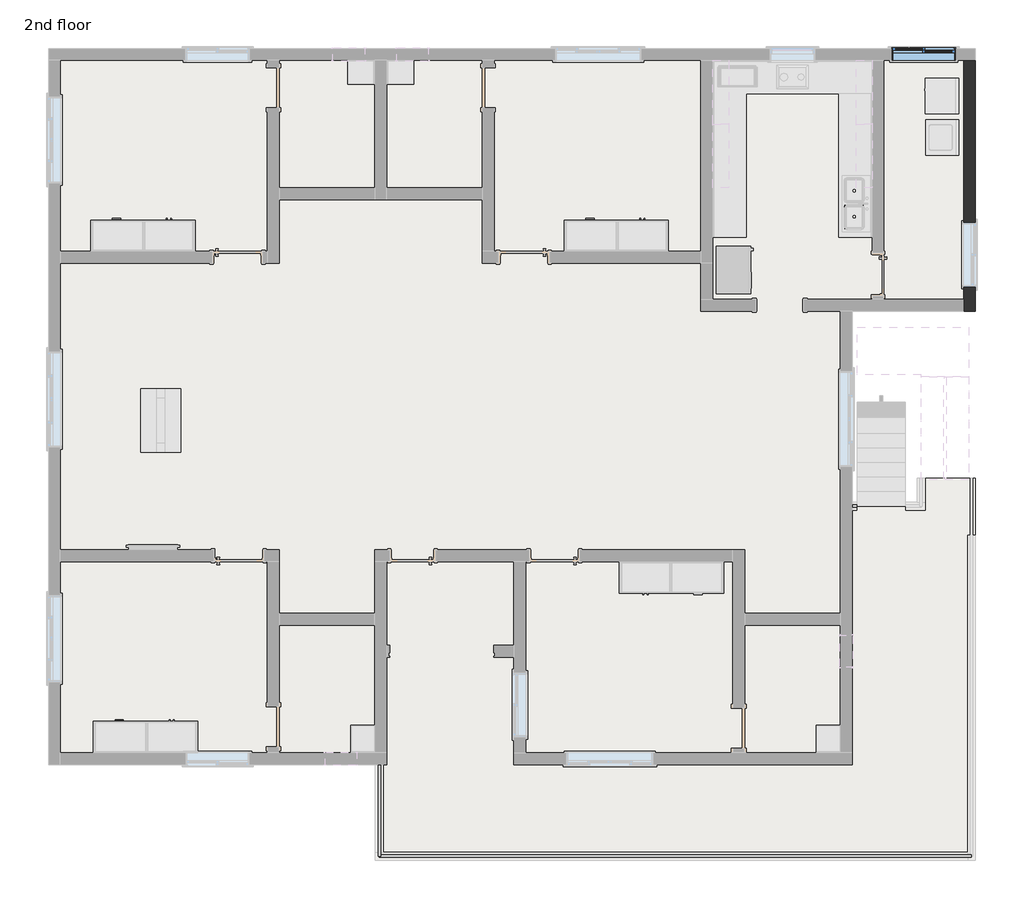
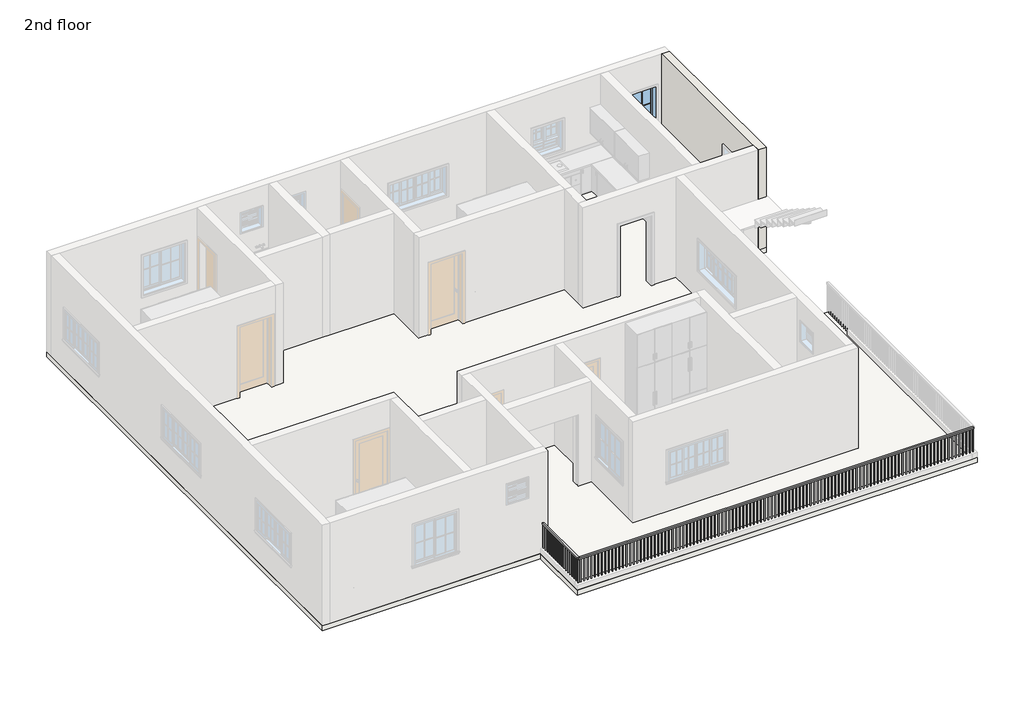
# One storey, part 2 of 4: 3 railings, 1 slab, 1 wall, 1 window.
"""IFC4 building model written with IfcOpenShell, lengths in millimetres."""

from ifc_helpers import new_model, si_unit, frame, origin, place, context, project, spatial, polyline, outline, extrude, faceted_brep, transform, mapped, element, save
from components import window_5af5dca6

model = new_model("IFC4")

# Units and contexts
model_context = context("Model", 3, world=origin())
ifc_project = project(units=[si_unit("LENGTHUNIT", "METRE", prefix="MILLI")], contexts=[model_context])

# Site, building, storey
site = spatial("IfcSite", under=ifc_project)
building = spatial("IfcBuilding", under=site)
storey = spatial("IfcBuildingStorey", under=building, Name="2nd floor", Elevation=7010.4)

# Railings
placement = place(None, origin())
element("IfcRailing", 1, ObjectType="Handrail - Rectangular", at=placement, inside=storey, context=model_context, shape_type="SweptSolid", body=[
    extrude(outline(polyline([(9648.8260838, -8369.2339187), (9648.8260838, -8420.0339187), (-1692.2739162, -8420.0339187), (-1692.2739162, -8369.2339187), (9648.8260838, -8369.2339187)])), frame((0.0, 0.0, 7874.0), z_axis=(0.0, 0.0, 1.0), x_axis=(1.0, 0.0, 0.0)), (0.0, 0.0, 1.0), 50.8),
    extrude(outline(polyline([(-1619.2489162, -8385.1089187), (-1619.2489162, -8404.1589187), (-1638.2989162, -8404.1589187), (-1638.2989162, -8385.1089187), (-1619.2489162, -8385.1089187)])), frame((0.0, 0.0, 7010.4), z_axis=(0.0, 0.0, 1.0), x_axis=(1.0, 0.0, 0.0)), (0.0, 0.0, 1.0), 863.6),
    extrude(outline(polyline([(-1517.6489162, -8385.1089187), (-1517.6489162, -8404.1589187), (-1536.6989162, -8404.1589187), (-1536.6989162, -8385.1089187), (-1517.6489162, -8385.1089187)])), frame((0.0, 0.0, 7010.4), z_axis=(0.0, 0.0, 1.0), x_axis=(1.0, 0.0, 0.0)), (0.0, 0.0, 1.0), 863.6),
    extrude(outline(polyline([(-1416.0489162, -8385.1089187), (-1416.0489162, -8404.1589187), (-1435.0989162, -8404.1589187), (-1435.0989162, -8385.1089187), (-1416.0489162, -8385.1089187)])), frame((0.0, 0.0, 7010.4), z_axis=(0.0, 0.0, 1.0), x_axis=(1.0, 0.0, 0.0)), (0.0, 0.0, 1.0), 863.6),
    extrude(outline(polyline([(-1314.4489162, -8385.1089187), (-1314.4489162, -8404.1589187), (-1333.4989162, -8404.1589187), (-1333.4989162, -8385.1089187), (-1314.4489162, -8385.1089187)])), frame((0.0, 0.0, 7010.4), z_axis=(0.0, 0.0, 1.0), x_axis=(1.0, 0.0, 0.0)), (0.0, 0.0, 1.0), 863.6),
    extrude(outline(polyline([(-1212.8489162, -8385.1089187), (-1212.8489162, -8404.1589187), (-1231.8989162, -8404.1589187), (-1231.8989162, -8385.1089187), (-1212.8489162, -8385.1089187)])), frame((0.0, 0.0, 7010.4), z_axis=(0.0, 0.0, 1.0), x_axis=(1.0, 0.0, 0.0)), (0.0, 0.0, 1.0), 863.6),
    extrude(outline(polyline([(-1111.2489162, -8385.1089187), (-1111.2489162, -8404.1589187), (-1130.2989162, -8404.1589187), (-1130.2989162, -8385.1089187), (-1111.2489162, -8385.1089187)])), frame((0.0, 0.0, 7010.4), z_axis=(0.0, 0.0, 1.0), x_axis=(1.0, 0.0, 0.0)), (0.0, 0.0, 1.0), 863.6),
    extrude(outline(polyline([(-1009.6489162, -8385.1089187), (-1009.6489162, -8404.1589187), (-1028.6989162, -8404.1589187), (-1028.6989162, -8385.1089187), (-1009.6489162, -8385.1089187)])), frame((0.0, 0.0, 7010.4), z_axis=(0.0, 0.0, 1.0), x_axis=(1.0, 0.0, 0.0)), (0.0, 0.0, 1.0), 863.6),
    extrude(outline(polyline([(-908.0489162, -8385.1089187), (-908.0489162, -8404.1589187), (-927.0989162, -8404.1589187), (-927.0989162, -8385.1089187), (-908.0489162, -8385.1089187)])), frame((0.0, 0.0, 7010.4), z_axis=(0.0, 0.0, 1.0), x_axis=(1.0, 0.0, 0.0)), (0.0, 0.0, 1.0), 863.6),
    extrude(outline(polyline([(-806.4489162, -8385.1089187), (-806.4489162, -8404.1589187), (-825.4989162, -8404.1589187), (-825.4989162, -8385.1089187), (-806.4489162, -8385.1089187)])), frame((0.0, 0.0, 7010.4), z_axis=(0.0, 0.0, 1.0), x_axis=(1.0, 0.0, 0.0)), (0.0, 0.0, 1.0), 863.6),
    extrude(outline(polyline([(-704.8489162, -8385.1089187), (-704.8489162, -8404.1589187), (-723.8989162, -8404.1589187), (-723.8989162, -8385.1089187), (-704.8489162, -8385.1089187)])), frame((0.0, 0.0, 7010.4), z_axis=(0.0, 0.0, 1.0), x_axis=(1.0, 0.0, 0.0)), (0.0, 0.0, 1.0), 863.6),
    extrude(outline(polyline([(-603.2489162, -8385.1089187), (-603.2489162, -8404.1589187), (-622.2989162, -8404.1589187), (-622.2989162, -8385.1089187), (-603.2489162, -8385.1089187)])), frame((0.0, 0.0, 7010.4), z_axis=(0.0, 0.0, 1.0), x_axis=(1.0, 0.0, 0.0)), (0.0, 0.0, 1.0), 863.6),
    extrude(outline(polyline([(-501.6489162, -8385.1089187), (-501.6489162, -8404.1589187), (-520.6989162, -8404.1589187), (-520.6989162, -8385.1089187), (-501.6489162, -8385.1089187)])), frame((0.0, 0.0, 7010.4), z_axis=(0.0, 0.0, 1.0), x_axis=(1.0, 0.0, 0.0)), (0.0, 0.0, 1.0), 863.6),
    extrude(outline(polyline([(-400.0489162, -8385.1089187), (-400.0489162, -8404.1589187), (-419.0989162, -8404.1589187), (-419.0989162, -8385.1089187), (-400.0489162, -8385.1089187)])), frame((0.0, 0.0, 7010.4), z_axis=(0.0, 0.0, 1.0), x_axis=(1.0, 0.0, 0.0)), (0.0, 0.0, 1.0), 863.6),
    extrude(outline(polyline([(-298.4489162, -8385.1089187), (-298.4489162, -8404.1589187), (-317.4989162, -8404.1589187), (-317.4989162, -8385.1089187), (-298.4489162, -8385.1089187)])), frame((0.0, 0.0, 7010.4), z_axis=(0.0, 0.0, 1.0), x_axis=(1.0, 0.0, 0.0)), (0.0, 0.0, 1.0), 863.6),
    extrude(outline(polyline([(-196.8489162, -8385.1089187), (-196.8489162, -8404.1589187), (-215.8989162, -8404.1589187), (-215.8989162, -8385.1089187), (-196.8489162, -8385.1089187)])), frame((0.0, 0.0, 7010.4), z_axis=(0.0, 0.0, 1.0), x_axis=(1.0, 0.0, 0.0)), (0.0, 0.0, 1.0), 863.6),
    extrude(outline(polyline([(-95.2489162, -8385.1089187), (-95.2489162, -8404.1589187), (-114.2989162, -8404.1589187), (-114.2989162, -8385.1089187), (-95.2489162, -8385.1089187)])), frame((0.0, 0.0, 7010.4), z_axis=(0.0, 0.0, 1.0), x_axis=(1.0, 0.0, 0.0)), (0.0, 0.0, 1.0), 863.6),
    extrude(outline(polyline([(6.3510838, -8385.1089187), (6.3510838, -8404.1589187), (-12.6989162, -8404.1589187), (-12.6989162, -8385.1089187), (6.3510838, -8385.1089187)])), frame((0.0, 0.0, 7010.4), z_axis=(0.0, 0.0, 1.0), x_axis=(1.0, 0.0, 0.0)), (0.0, 0.0, 1.0), 863.6),
    extrude(outline(polyline([(107.9510838, -8385.1089187), (107.9510838, -8404.1589187), (88.9010838, -8404.1589187), (88.9010838, -8385.1089187), (107.9510838, -8385.1089187)])), frame((0.0, 0.0, 7010.4), z_axis=(0.0, 0.0, 1.0), x_axis=(1.0, 0.0, 0.0)), (0.0, 0.0, 1.0), 863.6),
    extrude(outline(polyline([(209.5510838, -8385.1089187), (209.5510838, -8404.1589187), (190.5010838, -8404.1589187), (190.5010838, -8385.1089187), (209.5510838, -8385.1089187)])), frame((0.0, 0.0, 7010.4), z_axis=(0.0, 0.0, 1.0), x_axis=(1.0, 0.0, 0.0)), (0.0, 0.0, 1.0), 863.6),
    extrude(outline(polyline([(311.1510838, -8385.1089187), (311.1510838, -8404.1589187), (292.1010838, -8404.1589187), (292.1010838, -8385.1089187), (311.1510838, -8385.1089187)])), frame((0.0, 0.0, 7010.4), z_axis=(0.0, 0.0, 1.0), x_axis=(1.0, 0.0, 0.0)), (0.0, 0.0, 1.0), 863.6),
    extrude(outline(polyline([(412.7510838, -8385.1089187), (412.7510838, -8404.1589187), (393.7010838, -8404.1589187), (393.7010838, -8385.1089187), (412.7510838, -8385.1089187)])), frame((0.0, 0.0, 7010.4), z_axis=(0.0, 0.0, 1.0), x_axis=(1.0, 0.0, 0.0)), (0.0, 0.0, 1.0), 863.6),
    extrude(outline(polyline([(514.3510838, -8385.1089187), (514.3510838, -8404.1589187), (495.3010838, -8404.1589187), (495.3010838, -8385.1089187), (514.3510838, -8385.1089187)])), frame((0.0, 0.0, 7010.4), z_axis=(0.0, 0.0, 1.0), x_axis=(1.0, 0.0, 0.0)), (0.0, 0.0, 1.0), 863.6),
    extrude(outline(polyline([(615.9510838, -8385.1089187), (615.9510838, -8404.1589187), (596.9010838, -8404.1589187), (596.9010838, -8385.1089187), (615.9510838, -8385.1089187)])), frame((0.0, 0.0, 7010.4), z_axis=(0.0, 0.0, 1.0), x_axis=(1.0, 0.0, 0.0)), (0.0, 0.0, 1.0), 863.6),
    extrude(outline(polyline([(717.5510838, -8385.1089187), (717.5510838, -8404.1589187), (698.5010838, -8404.1589187), (698.5010838, -8385.1089187), (717.5510838, -8385.1089187)])), frame((0.0, 0.0, 7010.4), z_axis=(0.0, 0.0, 1.0), x_axis=(1.0, 0.0, 0.0)), (0.0, 0.0, 1.0), 863.6),
    extrude(outline(polyline([(819.1510838, -8385.1089187), (819.1510838, -8404.1589187), (800.1010838, -8404.1589187), (800.1010838, -8385.1089187), (819.1510838, -8385.1089187)])), frame((0.0, 0.0, 7010.4), z_axis=(0.0, 0.0, 1.0), x_axis=(1.0, 0.0, 0.0)), (0.0, 0.0, 1.0), 863.6),
    extrude(outline(polyline([(920.7510838, -8385.1089187), (920.7510838, -8404.1589187), (901.7010838, -8404.1589187), (901.7010838, -8385.1089187), (920.7510838, -8385.1089187)])), frame((0.0, 0.0, 7010.4), z_axis=(0.0, 0.0, 1.0), x_axis=(1.0, 0.0, 0.0)), (0.0, 0.0, 1.0), 863.6),
    extrude(outline(polyline([(1022.3510838, -8385.1089187), (1022.3510838, -8404.1589187), (1003.3010838, -8404.1589187), (1003.3010838, -8385.1089187), (1022.3510838, -8385.1089187)])), frame((0.0, 0.0, 7010.4), z_axis=(0.0, 0.0, 1.0), x_axis=(1.0, 0.0, 0.0)), (0.0, 0.0, 1.0), 863.6),
    extrude(outline(polyline([(1123.9510838, -8385.1089187), (1123.9510838, -8404.1589187), (1104.9010838, -8404.1589187), (1104.9010838, -8385.1089187), (1123.9510838, -8385.1089187)])), frame((0.0, 0.0, 7010.4), z_axis=(0.0, 0.0, 1.0), x_axis=(1.0, 0.0, 0.0)), (0.0, 0.0, 1.0), 863.6),
    extrude(outline(polyline([(1225.5510838, -8385.1089187), (1225.5510838, -8404.1589187), (1206.5010838, -8404.1589187), (1206.5010838, -8385.1089187), (1225.5510838, -8385.1089187)])), frame((0.0, 0.0, 7010.4), z_axis=(0.0, 0.0, 1.0), x_axis=(1.0, 0.0, 0.0)), (0.0, 0.0, 1.0), 863.6),
    extrude(outline(polyline([(1327.1510838, -8385.1089187), (1327.1510838, -8404.1589187), (1308.1010838, -8404.1589187), (1308.1010838, -8385.1089187), (1327.1510838, -8385.1089187)])), frame((0.0, 0.0, 7010.4), z_axis=(0.0, 0.0, 1.0), x_axis=(1.0, 0.0, 0.0)), (0.0, 0.0, 1.0), 863.6),
    extrude(outline(polyline([(1428.7510838, -8385.1089187), (1428.7510838, -8404.1589187), (1409.7010838, -8404.1589187), (1409.7010838, -8385.1089187), (1428.7510838, -8385.1089187)])), frame((0.0, 0.0, 7010.4), z_axis=(0.0, 0.0, 1.0), x_axis=(1.0, 0.0, 0.0)), (0.0, 0.0, 1.0), 863.6),
    extrude(outline(polyline([(1530.3510838, -8385.1089187), (1530.3510838, -8404.1589187), (1511.3010838, -8404.1589187), (1511.3010838, -8385.1089187), (1530.3510838, -8385.1089187)])), frame((0.0, 0.0, 7010.4), z_axis=(0.0, 0.0, 1.0), x_axis=(1.0, 0.0, 0.0)), (0.0, 0.0, 1.0), 863.6),
    extrude(outline(polyline([(1631.9510838, -8385.1089187), (1631.9510838, -8404.1589187), (1612.9010838, -8404.1589187), (1612.9010838, -8385.1089187), (1631.9510838, -8385.1089187)])), frame((0.0, 0.0, 7010.4), z_axis=(0.0, 0.0, 1.0), x_axis=(1.0, 0.0, 0.0)), (0.0, 0.0, 1.0), 863.6),
    extrude(outline(polyline([(1733.5510838, -8385.1089187), (1733.5510838, -8404.1589187), (1714.5010838, -8404.1589187), (1714.5010838, -8385.1089187), (1733.5510838, -8385.1089187)])), frame((0.0, 0.0, 7010.4), z_axis=(0.0, 0.0, 1.0), x_axis=(1.0, 0.0, 0.0)), (0.0, 0.0, 1.0), 863.6),
    extrude(outline(polyline([(1835.1510838, -8385.1089187), (1835.1510838, -8404.1589187), (1816.1010838, -8404.1589187), (1816.1010838, -8385.1089187), (1835.1510838, -8385.1089187)])), frame((0.0, 0.0, 7010.4), z_axis=(0.0, 0.0, 1.0), x_axis=(1.0, 0.0, 0.0)), (0.0, 0.0, 1.0), 863.6),
    extrude(outline(polyline([(1936.7510838, -8385.1089187), (1936.7510838, -8404.1589187), (1917.7010838, -8404.1589187), (1917.7010838, -8385.1089187), (1936.7510838, -8385.1089187)])), frame((0.0, 0.0, 7010.4), z_axis=(0.0, 0.0, 1.0), x_axis=(1.0, 0.0, 0.0)), (0.0, 0.0, 1.0), 863.6),
    extrude(outline(polyline([(2038.3510838, -8385.1089187), (2038.3510838, -8404.1589187), (2019.3010838, -8404.1589187), (2019.3010838, -8385.1089187), (2038.3510838, -8385.1089187)])), frame((0.0, 0.0, 7010.4), z_axis=(0.0, 0.0, 1.0), x_axis=(1.0, 0.0, 0.0)), (0.0, 0.0, 1.0), 863.6),
    extrude(outline(polyline([(2139.9510838, -8385.1089187), (2139.9510838, -8404.1589187), (2120.9010838, -8404.1589187), (2120.9010838, -8385.1089187), (2139.9510838, -8385.1089187)])), frame((0.0, 0.0, 7010.4), z_axis=(0.0, 0.0, 1.0), x_axis=(1.0, 0.0, 0.0)), (0.0, 0.0, 1.0), 863.6),
    extrude(outline(polyline([(2241.5510838, -8385.1089187), (2241.5510838, -8404.1589187), (2222.5010838, -8404.1589187), (2222.5010838, -8385.1089187), (2241.5510838, -8385.1089187)])), frame((0.0, 0.0, 7010.4), z_axis=(0.0, 0.0, 1.0), x_axis=(1.0, 0.0, 0.0)), (0.0, 0.0, 1.0), 863.6),
    extrude(outline(polyline([(2343.1510838, -8385.1089187), (2343.1510838, -8404.1589187), (2324.1010838, -8404.1589187), (2324.1010838, -8385.1089187), (2343.1510838, -8385.1089187)])), frame((0.0, 0.0, 7010.4), z_axis=(0.0, 0.0, 1.0), x_axis=(1.0, 0.0, 0.0)), (0.0, 0.0, 1.0), 863.6),
    extrude(outline(polyline([(2444.7510838, -8385.1089187), (2444.7510838, -8404.1589187), (2425.7010838, -8404.1589187), (2425.7010838, -8385.1089187), (2444.7510838, -8385.1089187)])), frame((0.0, 0.0, 7010.4), z_axis=(0.0, 0.0, 1.0), x_axis=(1.0, 0.0, 0.0)), (0.0, 0.0, 1.0), 863.6),
    extrude(outline(polyline([(2546.3510838, -8385.1089187), (2546.3510838, -8404.1589187), (2527.3010838, -8404.1589187), (2527.3010838, -8385.1089187), (2546.3510838, -8385.1089187)])), frame((0.0, 0.0, 7010.4), z_axis=(0.0, 0.0, 1.0), x_axis=(1.0, 0.0, 0.0)), (0.0, 0.0, 1.0), 863.6),
    extrude(outline(polyline([(2647.9510838, -8385.1089187), (2647.9510838, -8404.1589187), (2628.9010838, -8404.1589187), (2628.9010838, -8385.1089187), (2647.9510838, -8385.1089187)])), frame((0.0, 0.0, 7010.4), z_axis=(0.0, 0.0, 1.0), x_axis=(1.0, 0.0, 0.0)), (0.0, 0.0, 1.0), 863.6),
    extrude(outline(polyline([(2749.5510838, -8385.1089187), (2749.5510838, -8404.1589187), (2730.5010838, -8404.1589187), (2730.5010838, -8385.1089187), (2749.5510838, -8385.1089187)])), frame((0.0, 0.0, 7010.4), z_axis=(0.0, 0.0, 1.0), x_axis=(1.0, 0.0, 0.0)), (0.0, 0.0, 1.0), 863.6),
    extrude(outline(polyline([(2851.1510838, -8385.1089187), (2851.1510838, -8404.1589187), (2832.1010838, -8404.1589187), (2832.1010838, -8385.1089187), (2851.1510838, -8385.1089187)])), frame((0.0, 0.0, 7010.4), z_axis=(0.0, 0.0, 1.0), x_axis=(1.0, 0.0, 0.0)), (0.0, 0.0, 1.0), 863.6),
    extrude(outline(polyline([(2952.7510838, -8385.1089187), (2952.7510838, -8404.1589187), (2933.7010838, -8404.1589187), (2933.7010838, -8385.1089187), (2952.7510838, -8385.1089187)])), frame((0.0, 0.0, 7010.4), z_axis=(0.0, 0.0, 1.0), x_axis=(1.0, 0.0, 0.0)), (0.0, 0.0, 1.0), 863.6),
    extrude(outline(polyline([(3054.3510838, -8385.1089187), (3054.3510838, -8404.1589187), (3035.3010838, -8404.1589187), (3035.3010838, -8385.1089187), (3054.3510838, -8385.1089187)])), frame((0.0, 0.0, 7010.4), z_axis=(0.0, 0.0, 1.0), x_axis=(1.0, 0.0, 0.0)), (0.0, 0.0, 1.0), 863.6),
    extrude(outline(polyline([(3155.9510838, -8385.1089187), (3155.9510838, -8404.1589187), (3136.9010838, -8404.1589187), (3136.9010838, -8385.1089187), (3155.9510838, -8385.1089187)])), frame((0.0, 0.0, 7010.4), z_axis=(0.0, 0.0, 1.0), x_axis=(1.0, 0.0, 0.0)), (0.0, 0.0, 1.0), 863.6),
    extrude(outline(polyline([(3257.5510838, -8385.1089187), (3257.5510838, -8404.1589187), (3238.5010838, -8404.1589187), (3238.5010838, -8385.1089187), (3257.5510838, -8385.1089187)])), frame((0.0, 0.0, 7010.4), z_axis=(0.0, 0.0, 1.0), x_axis=(1.0, 0.0, 0.0)), (0.0, 0.0, 1.0), 863.6),
    extrude(outline(polyline([(3359.1510838, -8385.1089187), (3359.1510838, -8404.1589187), (3340.1010838, -8404.1589187), (3340.1010838, -8385.1089187), (3359.1510838, -8385.1089187)])), frame((0.0, 0.0, 7010.4), z_axis=(0.0, 0.0, 1.0), x_axis=(1.0, 0.0, 0.0)), (0.0, 0.0, 1.0), 863.6),
    extrude(outline(polyline([(3460.7510838, -8385.1089187), (3460.7510838, -8404.1589187), (3441.7010838, -8404.1589187), (3441.7010838, -8385.1089187), (3460.7510838, -8385.1089187)])), frame((0.0, 0.0, 7010.4), z_axis=(0.0, 0.0, 1.0), x_axis=(1.0, 0.0, 0.0)), (0.0, 0.0, 1.0), 863.6),
    extrude(outline(polyline([(3562.3510838, -8385.1089187), (3562.3510838, -8404.1589187), (3543.3010838, -8404.1589187), (3543.3010838, -8385.1089187), (3562.3510838, -8385.1089187)])), frame((0.0, 0.0, 7010.4), z_axis=(0.0, 0.0, 1.0), x_axis=(1.0, 0.0, 0.0)), (0.0, 0.0, 1.0), 863.6),
    extrude(outline(polyline([(3663.9510838, -8385.1089187), (3663.9510838, -8404.1589187), (3644.9010838, -8404.1589187), (3644.9010838, -8385.1089187), (3663.9510838, -8385.1089187)])), frame((0.0, 0.0, 7010.4), z_axis=(0.0, 0.0, 1.0), x_axis=(1.0, 0.0, 0.0)), (0.0, 0.0, 1.0), 863.6),
    extrude(outline(polyline([(3765.5510838, -8385.1089187), (3765.5510838, -8404.1589187), (3746.5010838, -8404.1589187), (3746.5010838, -8385.1089187), (3765.5510838, -8385.1089187)])), frame((0.0, 0.0, 7010.4), z_axis=(0.0, 0.0, 1.0), x_axis=(1.0, 0.0, 0.0)), (0.0, 0.0, 1.0), 863.6),
    extrude(outline(polyline([(3867.1510838, -8385.1089187), (3867.1510838, -8404.1589187), (3848.1010838, -8404.1589187), (3848.1010838, -8385.1089187), (3867.1510838, -8385.1089187)])), frame((0.0, 0.0, 7010.4), z_axis=(0.0, 0.0, 1.0), x_axis=(1.0, 0.0, 0.0)), (0.0, 0.0, 1.0), 863.6),
    extrude(outline(polyline([(3968.7510838, -8385.1089187), (3968.7510838, -8404.1589187), (3949.7010838, -8404.1589187), (3949.7010838, -8385.1089187), (3968.7510838, -8385.1089187)])), frame((0.0, 0.0, 7010.4), z_axis=(0.0, 0.0, 1.0), x_axis=(1.0, 0.0, 0.0)), (0.0, 0.0, 1.0), 863.6),
    extrude(outline(polyline([(4070.3510838, -8385.1089187), (4070.3510838, -8404.1589187), (4051.3010838, -8404.1589187), (4051.3010838, -8385.1089187), (4070.3510838, -8385.1089187)])), frame((0.0, 0.0, 7010.4), z_axis=(0.0, 0.0, 1.0), x_axis=(1.0, 0.0, 0.0)), (0.0, 0.0, 1.0), 863.6),
    extrude(outline(polyline([(4171.9510838, -8385.1089187), (4171.9510838, -8404.1589187), (4152.9010838, -8404.1589187), (4152.9010838, -8385.1089187), (4171.9510838, -8385.1089187)])), frame((0.0, 0.0, 7010.4), z_axis=(0.0, 0.0, 1.0), x_axis=(1.0, 0.0, 0.0)), (0.0, 0.0, 1.0), 863.6),
    extrude(outline(polyline([(4273.5510838, -8385.1089187), (4273.5510838, -8404.1589187), (4254.5010838, -8404.1589187), (4254.5010838, -8385.1089187), (4273.5510838, -8385.1089187)])), frame((0.0, 0.0, 7010.4), z_axis=(0.0, 0.0, 1.0), x_axis=(1.0, 0.0, 0.0)), (0.0, 0.0, 1.0), 863.6),
    extrude(outline(polyline([(4375.1510838, -8385.1089187), (4375.1510838, -8404.1589187), (4356.1010838, -8404.1589187), (4356.1010838, -8385.1089187), (4375.1510838, -8385.1089187)])), frame((0.0, 0.0, 7010.4), z_axis=(0.0, 0.0, 1.0), x_axis=(1.0, 0.0, 0.0)), (0.0, 0.0, 1.0), 863.6),
    extrude(outline(polyline([(4476.7510838, -8385.1089187), (4476.7510838, -8404.1589187), (4457.7010838, -8404.1589187), (4457.7010838, -8385.1089187), (4476.7510838, -8385.1089187)])), frame((0.0, 0.0, 7010.4), z_axis=(0.0, 0.0, 1.0), x_axis=(1.0, 0.0, 0.0)), (0.0, 0.0, 1.0), 863.6),
    extrude(outline(polyline([(4578.3510838, -8385.1089187), (4578.3510838, -8404.1589187), (4559.3010838, -8404.1589187), (4559.3010838, -8385.1089187), (4578.3510838, -8385.1089187)])), frame((0.0, 0.0, 7010.4), z_axis=(0.0, 0.0, 1.0), x_axis=(1.0, 0.0, 0.0)), (0.0, 0.0, 1.0), 863.6),
    extrude(outline(polyline([(4679.9510838, -8385.1089187), (4679.9510838, -8404.1589187), (4660.9010838, -8404.1589187), (4660.9010838, -8385.1089187), (4679.9510838, -8385.1089187)])), frame((0.0, 0.0, 7010.4), z_axis=(0.0, 0.0, 1.0), x_axis=(1.0, 0.0, 0.0)), (0.0, 0.0, 1.0), 863.6),
    extrude(outline(polyline([(4781.5510838, -8385.1089187), (4781.5510838, -8404.1589187), (4762.5010838, -8404.1589187), (4762.5010838, -8385.1089187), (4781.5510838, -8385.1089187)])), frame((0.0, 0.0, 7010.4), z_axis=(0.0, 0.0, 1.0), x_axis=(1.0, 0.0, 0.0)), (0.0, 0.0, 1.0), 863.6),
    extrude(outline(polyline([(4883.1510838, -8385.1089187), (4883.1510838, -8404.1589187), (4864.1010838, -8404.1589187), (4864.1010838, -8385.1089187), (4883.1510838, -8385.1089187)])), frame((0.0, 0.0, 7010.4), z_axis=(0.0, 0.0, 1.0), x_axis=(1.0, 0.0, 0.0)), (0.0, 0.0, 1.0), 863.6),
    extrude(outline(polyline([(4984.7510838, -8385.1089187), (4984.7510838, -8404.1589187), (4965.7010838, -8404.1589187), (4965.7010838, -8385.1089187), (4984.7510838, -8385.1089187)])), frame((0.0, 0.0, 7010.4), z_axis=(0.0, 0.0, 1.0), x_axis=(1.0, 0.0, 0.0)), (0.0, 0.0, 1.0), 863.6),
    extrude(outline(polyline([(5086.3510838, -8385.1089187), (5086.3510838, -8404.1589187), (5067.3010838, -8404.1589187), (5067.3010838, -8385.1089187), (5086.3510838, -8385.1089187)])), frame((0.0, 0.0, 7010.4), z_axis=(0.0, 0.0, 1.0), x_axis=(1.0, 0.0, 0.0)), (0.0, 0.0, 1.0), 863.6),
    extrude(outline(polyline([(5187.9510838, -8385.1089187), (5187.9510838, -8404.1589187), (5168.9010838, -8404.1589187), (5168.9010838, -8385.1089187), (5187.9510838, -8385.1089187)])), frame((0.0, 0.0, 7010.4), z_axis=(0.0, 0.0, 1.0), x_axis=(1.0, 0.0, 0.0)), (0.0, 0.0, 1.0), 863.6),
    extrude(outline(polyline([(5289.5510838, -8385.1089187), (5289.5510838, -8404.1589187), (5270.5010838, -8404.1589187), (5270.5010838, -8385.1089187), (5289.5510838, -8385.1089187)])), frame((0.0, 0.0, 7010.4), z_axis=(0.0, 0.0, 1.0), x_axis=(1.0, 0.0, 0.0)), (0.0, 0.0, 1.0), 863.6),
    extrude(outline(polyline([(5391.1510838, -8385.1089187), (5391.1510838, -8404.1589187), (5372.1010838, -8404.1589187), (5372.1010838, -8385.1089187), (5391.1510838, -8385.1089187)])), frame((0.0, 0.0, 7010.4), z_axis=(0.0, 0.0, 1.0), x_axis=(1.0, 0.0, 0.0)), (0.0, 0.0, 1.0), 863.6),
    extrude(outline(polyline([(5492.7510838, -8385.1089187), (5492.7510838, -8404.1589187), (5473.7010838, -8404.1589187), (5473.7010838, -8385.1089187), (5492.7510838, -8385.1089187)])), frame((0.0, 0.0, 7010.4), z_axis=(0.0, 0.0, 1.0), x_axis=(1.0, 0.0, 0.0)), (0.0, 0.0, 1.0), 863.6),
    extrude(outline(polyline([(5594.3510838, -8385.1089187), (5594.3510838, -8404.1589187), (5575.3010838, -8404.1589187), (5575.3010838, -8385.1089187), (5594.3510838, -8385.1089187)])), frame((0.0, 0.0, 7010.4), z_axis=(0.0, 0.0, 1.0), x_axis=(1.0, 0.0, 0.0)), (0.0, 0.0, 1.0), 863.6),
    extrude(outline(polyline([(5695.9510838, -8385.1089187), (5695.9510838, -8404.1589187), (5676.9010838, -8404.1589187), (5676.9010838, -8385.1089187), (5695.9510838, -8385.1089187)])), frame((0.0, 0.0, 7010.4), z_axis=(0.0, 0.0, 1.0), x_axis=(1.0, 0.0, 0.0)), (0.0, 0.0, 1.0), 863.6),
    extrude(outline(polyline([(5797.5510838, -8385.1089187), (5797.5510838, -8404.1589187), (5778.5010838, -8404.1589187), (5778.5010838, -8385.1089187), (5797.5510838, -8385.1089187)])), frame((0.0, 0.0, 7010.4), z_axis=(0.0, 0.0, 1.0), x_axis=(1.0, 0.0, 0.0)), (0.0, 0.0, 1.0), 863.6),
    extrude(outline(polyline([(5899.1510838, -8385.1089187), (5899.1510838, -8404.1589187), (5880.1010838, -8404.1589187), (5880.1010838, -8385.1089187), (5899.1510838, -8385.1089187)])), frame((0.0, 0.0, 7010.4), z_axis=(0.0, 0.0, 1.0), x_axis=(1.0, 0.0, 0.0)), (0.0, 0.0, 1.0), 863.6),
    extrude(outline(polyline([(6000.7510838, -8385.1089187), (6000.7510838, -8404.1589187), (5981.7010838, -8404.1589187), (5981.7010838, -8385.1089187), (6000.7510838, -8385.1089187)])), frame((0.0, 0.0, 7010.4), z_axis=(0.0, 0.0, 1.0), x_axis=(1.0, 0.0, 0.0)), (0.0, 0.0, 1.0), 863.6),
    extrude(outline(polyline([(6102.3510838, -8385.1089187), (6102.3510838, -8404.1589187), (6083.3010838, -8404.1589187), (6083.3010838, -8385.1089187), (6102.3510838, -8385.1089187)])), frame((0.0, 0.0, 7010.4), z_axis=(0.0, 0.0, 1.0), x_axis=(1.0, 0.0, 0.0)), (0.0, 0.0, 1.0), 863.6),
    extrude(outline(polyline([(6203.9510838, -8385.1089187), (6203.9510838, -8404.1589187), (6184.9010838, -8404.1589187), (6184.9010838, -8385.1089187), (6203.9510838, -8385.1089187)])), frame((0.0, 0.0, 7010.4), z_axis=(0.0, 0.0, 1.0), x_axis=(1.0, 0.0, 0.0)), (0.0, 0.0, 1.0), 863.6),
    extrude(outline(polyline([(6305.5510838, -8385.1089187), (6305.5510838, -8404.1589187), (6286.5010838, -8404.1589187), (6286.5010838, -8385.1089187), (6305.5510838, -8385.1089187)])), frame((0.0, 0.0, 7010.4), z_axis=(0.0, 0.0, 1.0), x_axis=(1.0, 0.0, 0.0)), (0.0, 0.0, 1.0), 863.6),
    extrude(outline(polyline([(6407.1510838, -8385.1089187), (6407.1510838, -8404.1589187), (6388.1010838, -8404.1589187), (6388.1010838, -8385.1089187), (6407.1510838, -8385.1089187)])), frame((0.0, 0.0, 7010.4), z_axis=(0.0, 0.0, 1.0), x_axis=(1.0, 0.0, 0.0)), (0.0, 0.0, 1.0), 863.6),
    extrude(outline(polyline([(6508.7510838, -8385.1089187), (6508.7510838, -8404.1589187), (6489.7010838, -8404.1589187), (6489.7010838, -8385.1089187), (6508.7510838, -8385.1089187)])), frame((0.0, 0.0, 7010.4), z_axis=(0.0, 0.0, 1.0), x_axis=(1.0, 0.0, 0.0)), (0.0, 0.0, 1.0), 863.6),
    extrude(outline(polyline([(6610.3510838, -8385.1089187), (6610.3510838, -8404.1589187), (6591.3010838, -8404.1589187), (6591.3010838, -8385.1089187), (6610.3510838, -8385.1089187)])), frame((0.0, 0.0, 7010.4), z_axis=(0.0, 0.0, 1.0), x_axis=(1.0, 0.0, 0.0)), (0.0, 0.0, 1.0), 863.6),
    extrude(outline(polyline([(6711.9510838, -8385.1089187), (6711.9510838, -8404.1589187), (6692.9010838, -8404.1589187), (6692.9010838, -8385.1089187), (6711.9510838, -8385.1089187)])), frame((0.0, 0.0, 7010.4), z_axis=(0.0, 0.0, 1.0), x_axis=(1.0, 0.0, 0.0)), (0.0, 0.0, 1.0), 863.6),
    extrude(outline(polyline([(6813.5510838, -8385.1089187), (6813.5510838, -8404.1589187), (6794.5010838, -8404.1589187), (6794.5010838, -8385.1089187), (6813.5510838, -8385.1089187)])), frame((0.0, 0.0, 7010.4), z_axis=(0.0, 0.0, 1.0), x_axis=(1.0, 0.0, 0.0)), (0.0, 0.0, 1.0), 863.6),
    extrude(outline(polyline([(6915.1510838, -8385.1089187), (6915.1510838, -8404.1589187), (6896.1010838, -8404.1589187), (6896.1010838, -8385.1089187), (6915.1510838, -8385.1089187)])), frame((0.0, 0.0, 7010.4), z_axis=(0.0, 0.0, 1.0), x_axis=(1.0, 0.0, 0.0)), (0.0, 0.0, 1.0), 863.6),
    extrude(outline(polyline([(7016.7510838, -8385.1089187), (7016.7510838, -8404.1589187), (6997.7010838, -8404.1589187), (6997.7010838, -8385.1089187), (7016.7510838, -8385.1089187)])), frame((0.0, 0.0, 7010.4), z_axis=(0.0, 0.0, 1.0), x_axis=(1.0, 0.0, 0.0)), (0.0, 0.0, 1.0), 863.6),
    extrude(outline(polyline([(7118.3510838, -8385.1089187), (7118.3510838, -8404.1589187), (7099.3010838, -8404.1589187), (7099.3010838, -8385.1089187), (7118.3510838, -8385.1089187)])), frame((0.0, 0.0, 7010.4), z_axis=(0.0, 0.0, 1.0), x_axis=(1.0, 0.0, 0.0)), (0.0, 0.0, 1.0), 863.6),
    extrude(outline(polyline([(7219.9510838, -8385.1089187), (7219.9510838, -8404.1589187), (7200.9010838, -8404.1589187), (7200.9010838, -8385.1089187), (7219.9510838, -8385.1089187)])), frame((0.0, 0.0, 7010.4), z_axis=(0.0, 0.0, 1.0), x_axis=(1.0, 0.0, 0.0)), (0.0, 0.0, 1.0), 863.6),
    extrude(outline(polyline([(7321.5510838, -8385.1089187), (7321.5510838, -8404.1589187), (7302.5010838, -8404.1589187), (7302.5010838, -8385.1089187), (7321.5510838, -8385.1089187)])), frame((0.0, 0.0, 7010.4), z_axis=(0.0, 0.0, 1.0), x_axis=(1.0, 0.0, 0.0)), (0.0, 0.0, 1.0), 863.6),
    extrude(outline(polyline([(7423.1510838, -8385.1089187), (7423.1510838, -8404.1589187), (7404.1010838, -8404.1589187), (7404.1010838, -8385.1089187), (7423.1510838, -8385.1089187)])), frame((0.0, 0.0, 7010.4), z_axis=(0.0, 0.0, 1.0), x_axis=(1.0, 0.0, 0.0)), (0.0, 0.0, 1.0), 863.6),
    extrude(outline(polyline([(7524.7510838, -8385.1089187), (7524.7510838, -8404.1589187), (7505.7010838, -8404.1589187), (7505.7010838, -8385.1089187), (7524.7510838, -8385.1089187)])), frame((0.0, 0.0, 7010.4), z_axis=(0.0, 0.0, 1.0), x_axis=(1.0, 0.0, 0.0)), (0.0, 0.0, 1.0), 863.6),
    extrude(outline(polyline([(7626.3510838, -8385.1089187), (7626.3510838, -8404.1589187), (7607.3010838, -8404.1589187), (7607.3010838, -8385.1089187), (7626.3510838, -8385.1089187)])), frame((0.0, 0.0, 7010.4), z_axis=(0.0, 0.0, 1.0), x_axis=(1.0, 0.0, 0.0)), (0.0, 0.0, 1.0), 863.6),
    extrude(outline(polyline([(7727.9510838, -8385.1089187), (7727.9510838, -8404.1589187), (7708.9010838, -8404.1589187), (7708.9010838, -8385.1089187), (7727.9510838, -8385.1089187)])), frame((0.0, 0.0, 7010.4), z_axis=(0.0, 0.0, 1.0), x_axis=(1.0, 0.0, 0.0)), (0.0, 0.0, 1.0), 863.6),
    extrude(outline(polyline([(7829.5510838, -8385.1089187), (7829.5510838, -8404.1589187), (7810.5010838, -8404.1589187), (7810.5010838, -8385.1089187), (7829.5510838, -8385.1089187)])), frame((0.0, 0.0, 7010.4), z_axis=(0.0, 0.0, 1.0), x_axis=(1.0, 0.0, 0.0)), (0.0, 0.0, 1.0), 863.6),
    extrude(outline(polyline([(7931.1510838, -8385.1089187), (7931.1510838, -8404.1589187), (7912.1010838, -8404.1589187), (7912.1010838, -8385.1089187), (7931.1510838, -8385.1089187)])), frame((0.0, 0.0, 7010.4), z_axis=(0.0, 0.0, 1.0), x_axis=(1.0, 0.0, 0.0)), (0.0, 0.0, 1.0), 863.6),
    extrude(outline(polyline([(8032.7510838, -8385.1089187), (8032.7510838, -8404.1589187), (8013.7010838, -8404.1589187), (8013.7010838, -8385.1089187), (8032.7510838, -8385.1089187)])), frame((0.0, 0.0, 7010.4), z_axis=(0.0, 0.0, 1.0), x_axis=(1.0, 0.0, 0.0)), (0.0, 0.0, 1.0), 863.6),
    extrude(outline(polyline([(8134.3510838, -8385.1089187), (8134.3510838, -8404.1589187), (8115.3010838, -8404.1589187), (8115.3010838, -8385.1089187), (8134.3510838, -8385.1089187)])), frame((0.0, 0.0, 7010.4), z_axis=(0.0, 0.0, 1.0), x_axis=(1.0, 0.0, 0.0)), (0.0, 0.0, 1.0), 863.6),
    extrude(outline(polyline([(8235.9510838, -8385.1089187), (8235.9510838, -8404.1589187), (8216.9010838, -8404.1589187), (8216.9010838, -8385.1089187), (8235.9510838, -8385.1089187)])), frame((0.0, 0.0, 7010.4), z_axis=(0.0, 0.0, 1.0), x_axis=(1.0, 0.0, 0.0)), (0.0, 0.0, 1.0), 863.6),
    extrude(outline(polyline([(8337.5510838, -8385.1089187), (8337.5510838, -8404.1589187), (8318.5010838, -8404.1589187), (8318.5010838, -8385.1089187), (8337.5510838, -8385.1089187)])), frame((0.0, 0.0, 7010.4), z_axis=(0.0, 0.0, 1.0), x_axis=(1.0, 0.0, 0.0)), (0.0, 0.0, 1.0), 863.6),
    extrude(outline(polyline([(8439.1510838, -8385.1089187), (8439.1510838, -8404.1589187), (8420.1010838, -8404.1589187), (8420.1010838, -8385.1089187), (8439.1510838, -8385.1089187)])), frame((0.0, 0.0, 7010.4), z_axis=(0.0, 0.0, 1.0), x_axis=(1.0, 0.0, 0.0)), (0.0, 0.0, 1.0), 863.6),
    extrude(outline(polyline([(8540.7510838, -8385.1089187), (8540.7510838, -8404.1589187), (8521.7010838, -8404.1589187), (8521.7010838, -8385.1089187), (8540.7510838, -8385.1089187)])), frame((0.0, 0.0, 7010.4), z_axis=(0.0, 0.0, 1.0), x_axis=(1.0, 0.0, 0.0)), (0.0, 0.0, 1.0), 863.6),
    extrude(outline(polyline([(8642.3510838, -8385.1089187), (8642.3510838, -8404.1589187), (8623.3010838, -8404.1589187), (8623.3010838, -8385.1089187), (8642.3510838, -8385.1089187)])), frame((0.0, 0.0, 7010.4), z_axis=(0.0, 0.0, 1.0), x_axis=(1.0, 0.0, 0.0)), (0.0, 0.0, 1.0), 863.6),
    extrude(outline(polyline([(8743.9510838, -8385.1089187), (8743.9510838, -8404.1589187), (8724.9010838, -8404.1589187), (8724.9010838, -8385.1089187), (8743.9510838, -8385.1089187)])), frame((0.0, 0.0, 7010.4), z_axis=(0.0, 0.0, 1.0), x_axis=(1.0, 0.0, 0.0)), (0.0, 0.0, 1.0), 863.6),
    extrude(outline(polyline([(8845.5510838, -8385.1089187), (8845.5510838, -8404.1589187), (8826.5010838, -8404.1589187), (8826.5010838, -8385.1089187), (8845.5510838, -8385.1089187)])), frame((0.0, 0.0, 7010.4), z_axis=(0.0, 0.0, 1.0), x_axis=(1.0, 0.0, 0.0)), (0.0, 0.0, 1.0), 863.6),
    extrude(outline(polyline([(8947.1510838, -8385.1089187), (8947.1510838, -8404.1589187), (8928.1010838, -8404.1589187), (8928.1010838, -8385.1089187), (8947.1510838, -8385.1089187)])), frame((0.0, 0.0, 7010.4), z_axis=(0.0, 0.0, 1.0), x_axis=(1.0, 0.0, 0.0)), (0.0, 0.0, 1.0), 863.6),
    extrude(outline(polyline([(9048.7510838, -8385.1089187), (9048.7510838, -8404.1589187), (9029.7010838, -8404.1589187), (9029.7010838, -8385.1089187), (9048.7510838, -8385.1089187)])), frame((0.0, 0.0, 7010.4), z_axis=(0.0, 0.0, 1.0), x_axis=(1.0, 0.0, 0.0)), (0.0, 0.0, 1.0), 863.6),
    extrude(outline(polyline([(9150.3510838, -8385.1089187), (9150.3510838, -8404.1589187), (9131.3010838, -8404.1589187), (9131.3010838, -8385.1089187), (9150.3510838, -8385.1089187)])), frame((0.0, 0.0, 7010.4), z_axis=(0.0, 0.0, 1.0), x_axis=(1.0, 0.0, 0.0)), (0.0, 0.0, 1.0), 863.6),
    extrude(outline(polyline([(9251.9510838, -8385.1089187), (9251.9510838, -8404.1589187), (9232.9010838, -8404.1589187), (9232.9010838, -8385.1089187), (9251.9510838, -8385.1089187)])), frame((0.0, 0.0, 7010.4), z_axis=(0.0, 0.0, 1.0), x_axis=(1.0, 0.0, 0.0)), (0.0, 0.0, 1.0), 863.6),
    extrude(outline(polyline([(9353.5510838, -8385.1089187), (9353.5510838, -8404.1589187), (9334.5010838, -8404.1589187), (9334.5010838, -8385.1089187), (9353.5510838, -8385.1089187)])), frame((0.0, 0.0, 7010.4), z_axis=(0.0, 0.0, 1.0), x_axis=(1.0, 0.0, 0.0)), (0.0, 0.0, 1.0), 863.6),
    extrude(outline(polyline([(9455.1510838, -8385.1089187), (9455.1510838, -8404.1589187), (9436.1010838, -8404.1589187), (9436.1010838, -8385.1089187), (9455.1510838, -8385.1089187)])), frame((0.0, 0.0, 7010.4), z_axis=(0.0, 0.0, 1.0), x_axis=(1.0, 0.0, 0.0)), (0.0, 0.0, 1.0), 863.6),
    extrude(outline(polyline([(9556.7510838, -8385.1089187), (9556.7510838, -8404.1589187), (9537.7010838, -8404.1589187), (9537.7010838, -8385.1089187), (9556.7510838, -8385.1089187)])), frame((0.0, 0.0, 7010.4), z_axis=(0.0, 0.0, 1.0), x_axis=(1.0, 0.0, 0.0)), (0.0, 0.0, 1.0), 863.6),
    extrude(outline(polyline([(-1673.2239162, -8385.1089187), (-1673.2239162, -8404.1589187), (-1692.2739162, -8404.1589187), (-1692.2739162, -8385.1089187), (-1673.2239162, -8385.1089187)])), frame((0.0, 0.0, 7010.4), z_axis=(0.0, 0.0, 1.0), x_axis=(1.0, 0.0, 0.0)), (0.0, 0.0, 1.0), 863.6),
    extrude(outline(polyline([(9648.8260838, -8385.1089187), (9648.8260838, -8404.1589187), (9629.7760838, -8404.1589187), (9629.7760838, -8385.1089187), (9648.8260838, -8385.1089187)])), frame((0.0, 0.0, 7010.4), z_axis=(0.0, 0.0, 1.0), x_axis=(1.0, 0.0, 0.0)), (0.0, 0.0, 1.0), 863.6),
])
element("IfcRailing", 2, ObjectType="Handrail - Rectangular", at=placement, inside=storey, context=model_context, shape_type="SweptSolid", body=[
    extrude(outline(polyline([(-1666.8739162, -8394.6339187), (-1717.6739162, -8394.6339187), (-1717.6739162, -6642.0339187), (-1666.8739162, -6642.0339187), (-1666.8739162, -8394.6339187)])), frame((0.0, 0.0, 7874.0), z_axis=(0.0, 0.0, 1.0), x_axis=(1.0, 0.0, 0.0)), (0.0, 0.0, 1.0), 50.8),
    extrude(outline(polyline([(-1682.7489162, -6676.9589187), (-1701.7989162, -6676.9589187), (-1701.7989162, -6657.9089187), (-1682.7489162, -6657.9089187), (-1682.7489162, -6676.9589187)])), frame((0.0, 0.0, 7010.4), z_axis=(0.0, 0.0, 1.0), x_axis=(1.0, 0.0, 0.0)), (0.0, 0.0, 1.0), 863.6),
    extrude(outline(polyline([(-1682.7489162, -6778.5589187), (-1701.7989162, -6778.5589187), (-1701.7989162, -6759.5089187), (-1682.7489162, -6759.5089187), (-1682.7489162, -6778.5589187)])), frame((0.0, 0.0, 7010.4), z_axis=(0.0, 0.0, 1.0), x_axis=(1.0, 0.0, 0.0)), (0.0, 0.0, 1.0), 863.6),
    extrude(outline(polyline([(-1682.7489162, -6880.1589187), (-1701.7989162, -6880.1589187), (-1701.7989162, -6861.1089187), (-1682.7489162, -6861.1089187), (-1682.7489162, -6880.1589187)])), frame((0.0, 0.0, 7010.4), z_axis=(0.0, 0.0, 1.0), x_axis=(1.0, 0.0, 0.0)), (0.0, 0.0, 1.0), 863.6),
    extrude(outline(polyline([(-1682.7489162, -6981.7589187), (-1701.7989162, -6981.7589187), (-1701.7989162, -6962.7089187), (-1682.7489162, -6962.7089187), (-1682.7489162, -6981.7589187)])), frame((0.0, 0.0, 7010.4), z_axis=(0.0, 0.0, 1.0), x_axis=(1.0, 0.0, 0.0)), (0.0, 0.0, 1.0), 863.6),
    extrude(outline(polyline([(-1682.7489162, -7083.3589187), (-1701.7989162, -7083.3589187), (-1701.7989162, -7064.3089187), (-1682.7489162, -7064.3089187), (-1682.7489162, -7083.3589187)])), frame((0.0, 0.0, 7010.4), z_axis=(0.0, 0.0, 1.0), x_axis=(1.0, 0.0, 0.0)), (0.0, 0.0, 1.0), 863.6),
    extrude(outline(polyline([(-1682.7489162, -7184.9589187), (-1701.7989162, -7184.9589187), (-1701.7989162, -7165.9089187), (-1682.7489162, -7165.9089187), (-1682.7489162, -7184.9589187)])), frame((0.0, 0.0, 7010.4), z_axis=(0.0, 0.0, 1.0), x_axis=(1.0, 0.0, 0.0)), (0.0, 0.0, 1.0), 863.6),
    extrude(outline(polyline([(-1682.7489162, -7286.5589187), (-1701.7989162, -7286.5589187), (-1701.7989162, -7267.5089187), (-1682.7489162, -7267.5089187), (-1682.7489162, -7286.5589187)])), frame((0.0, 0.0, 7010.4), z_axis=(0.0, 0.0, 1.0), x_axis=(1.0, 0.0, 0.0)), (0.0, 0.0, 1.0), 863.6),
    extrude(outline(polyline([(-1682.7489162, -7388.1589187), (-1701.7989162, -7388.1589187), (-1701.7989162, -7369.1089187), (-1682.7489162, -7369.1089187), (-1682.7489162, -7388.1589187)])), frame((0.0, 0.0, 7010.4), z_axis=(0.0, 0.0, 1.0), x_axis=(1.0, 0.0, 0.0)), (0.0, 0.0, 1.0), 863.6),
    extrude(outline(polyline([(-1682.7489162, -7489.7589187), (-1701.7989162, -7489.7589187), (-1701.7989162, -7470.7089187), (-1682.7489162, -7470.7089187), (-1682.7489162, -7489.7589187)])), frame((0.0, 0.0, 7010.4), z_axis=(0.0, 0.0, 1.0), x_axis=(1.0, 0.0, 0.0)), (0.0, 0.0, 1.0), 863.6),
    extrude(outline(polyline([(-1682.7489162, -7591.3589187), (-1701.7989162, -7591.3589187), (-1701.7989162, -7572.3089187), (-1682.7489162, -7572.3089187), (-1682.7489162, -7591.3589187)])), frame((0.0, 0.0, 7010.4), z_axis=(0.0, 0.0, 1.0), x_axis=(1.0, 0.0, 0.0)), (0.0, 0.0, 1.0), 863.6),
    extrude(outline(polyline([(-1682.7489162, -7692.9589187), (-1701.7989162, -7692.9589187), (-1701.7989162, -7673.9089187), (-1682.7489162, -7673.9089187), (-1682.7489162, -7692.9589187)])), frame((0.0, 0.0, 7010.4), z_axis=(0.0, 0.0, 1.0), x_axis=(1.0, 0.0, 0.0)), (0.0, 0.0, 1.0), 863.6),
    extrude(outline(polyline([(-1682.7489162, -7794.5589187), (-1701.7989162, -7794.5589187), (-1701.7989162, -7775.5089187), (-1682.7489162, -7775.5089187), (-1682.7489162, -7794.5589187)])), frame((0.0, 0.0, 7010.4), z_axis=(0.0, 0.0, 1.0), x_axis=(1.0, 0.0, 0.0)), (0.0, 0.0, 1.0), 863.6),
    extrude(outline(polyline([(-1682.7489162, -7896.1589187), (-1701.7989162, -7896.1589187), (-1701.7989162, -7877.1089187), (-1682.7489162, -7877.1089187), (-1682.7489162, -7896.1589187)])), frame((0.0, 0.0, 7010.4), z_axis=(0.0, 0.0, 1.0), x_axis=(1.0, 0.0, 0.0)), (0.0, 0.0, 1.0), 863.6),
    extrude(outline(polyline([(-1682.7489162, -7997.7589187), (-1701.7989162, -7997.7589187), (-1701.7989162, -7978.7089187), (-1682.7489162, -7978.7089187), (-1682.7489162, -7997.7589187)])), frame((0.0, 0.0, 7010.4), z_axis=(0.0, 0.0, 1.0), x_axis=(1.0, 0.0, 0.0)), (0.0, 0.0, 1.0), 863.6),
    extrude(outline(polyline([(-1682.7489162, -8099.3589187), (-1701.7989162, -8099.3589187), (-1701.7989162, -8080.3089187), (-1682.7489162, -8080.3089187), (-1682.7489162, -8099.3589187)])), frame((0.0, 0.0, 7010.4), z_axis=(0.0, 0.0, 1.0), x_axis=(1.0, 0.0, 0.0)), (0.0, 0.0, 1.0), 863.6),
    extrude(outline(polyline([(-1682.7489162, -8200.9589187), (-1701.7989162, -8200.9589187), (-1701.7989162, -8181.9089187), (-1682.7489162, -8181.9089187), (-1682.7489162, -8200.9589187)])), frame((0.0, 0.0, 7010.4), z_axis=(0.0, 0.0, 1.0), x_axis=(1.0, 0.0, 0.0)), (0.0, 0.0, 1.0), 863.6),
    extrude(outline(polyline([(-1682.7489162, -8302.5589187), (-1701.7989162, -8302.5589187), (-1701.7989162, -8283.5089187), (-1682.7489162, -8283.5089187), (-1682.7489162, -8302.5589187)])), frame((0.0, 0.0, 7010.4), z_axis=(0.0, 0.0, 1.0), x_axis=(1.0, 0.0, 0.0)), (0.0, 0.0, 1.0), 863.6),
    extrude(outline(polyline([(-1682.7489162, -6661.0839187), (-1701.7989162, -6661.0839187), (-1701.7989162, -6642.0339187), (-1682.7489162, -6642.0339187), (-1682.7489162, -6661.0839187)])), frame((0.0, 0.0, 7010.4), z_axis=(0.0, 0.0, 1.0), x_axis=(1.0, 0.0, 0.0)), (0.0, 0.0, 1.0), 863.6),
    extrude(outline(polyline([(-1682.7489162, -8394.6339187), (-1701.7989162, -8394.6339187), (-1701.7989162, -8375.5839187), (-1682.7489162, -8375.5839187), (-1682.7489162, -8394.6339187)])), frame((0.0, 0.0, 7010.4), z_axis=(0.0, 0.0, 1.0), x_axis=(1.0, 0.0, 0.0)), (0.0, 0.0, 1.0), 863.6),
])
element("IfcRailing", 3, ObjectType="Handrail - Rectangular", at=placement, inside=storey, context=model_context, shape_type="SweptSolid", body=[
    extrude(outline(polyline([(7451.7260838, -1663.6339187), (7451.7260838, -1714.4339187), (7362.8260838, -1714.4339187), (7362.8260838, -1663.6339187), (7451.7260838, -1663.6339187)])), frame((0.0, 0.0, 7874.0), z_axis=(0.0, 0.0, 1.0), x_axis=(1.0, 0.0, 0.0)), (0.0, 0.0, 1.0), 50.8),
    extrude(outline(polyline([(7381.8760838, -1679.5089187), (7381.8760838, -1698.5589187), (7362.8260838, -1698.5589187), (7362.8260838, -1679.5089187), (7381.8760838, -1679.5089187)])), frame((0.0, 0.0, 7010.4), z_axis=(0.0, 0.0, 1.0), x_axis=(1.0, 0.0, 0.0)), (0.0, 0.0, 1.0), 863.6),
    extrude(outline(polyline([(7451.7260838, -1679.5089187), (7451.7260838, -1698.5589187), (7432.6760838, -1698.5589187), (7432.6760838, -1679.5089187), (7451.7260838, -1679.5089187)])), frame((0.0, 0.0, 7010.4), z_axis=(0.0, 0.0, 1.0), x_axis=(1.0, 0.0, 0.0)), (0.0, 0.0, 1.0), 863.6),
])

# Slab
element("IfcSlab", 4, ObjectType="Generic - 6\"", at=placement, inside=storey, context=model_context, shape_type="SweptSolid", body=[
    extrude(outline(polyline([(-8029.5739162, 7073.9660813), (9725.0260838, 7073.9660813), (9725.0260838, 2044.7660813), (7362.8260838, 2044.7660813), (7362.8260838, -1689.0339187), (8683.6260838, -1689.0339187), (8683.6260838, -1155.6339187), (9725.0260838, -1155.6339187), (9725.0260838, -8470.8339187), (-1768.4739162, -8470.8339187), (-1768.4739162, -6642.0339187), (-8029.5739162, -6642.0339187), (-8029.5739162, 7073.9660813)])), frame((0.0, 0.0, 6858.0), z_axis=(0.0, 0.0, 1.0), x_axis=(1.0, 0.0, 0.0)), (0.0, 0.0, 1.0), 152.4),
])

# Wall
element("IfcWall", 5, ObjectType="Generic - 9\"", at=placement, inside=storey, context=model_context, shape_type="Brep", body=[
    faceted_brep([(9496.4260838, 6845.3660813, 7010.4), (9496.4260838, 2273.3660813, 7010.4), (9496.4260838, 2044.7660813, 7010.4), (9496.4260838, 2044.7660813, 10058.4), (9496.4260838, 2273.3660813, 10058.4), (9496.4260838, 6845.3660813, 10058.4), (9496.4260838, 2514.6660813, 9144.0), (9496.4260838, 2514.6660813, 7924.8), (9496.4260838, 3733.8660813, 7924.8), (9496.4260838, 3733.8660813, 9144.0), (9725.0260838, 2044.7660813, 7010.4), (9725.0260838, 6845.3660813, 7010.4), (9725.0260838, 6845.3660813, 10058.4), (9725.0260838, 2044.7660813, 10058.4), (9725.0260838, 2514.6660813, 7924.8), (9725.0260838, 2514.6660813, 9144.0), (9725.0260838, 3733.8660813, 9144.0), (9725.0260838, 3733.8660813, 7924.8)], [[[0, 1, 2, 3, 4, 5], [6, 7, 8, 9]], [[10, 11, 12, 13], [14, 15, 16, 17]], [[2, 1, 0, 11, 10]], [[3, 2, 10, 13]], [[0, 5, 12, 11]], [[6, 15, 14, 7]], [[7, 14, 17, 8]], [[8, 17, 16, 9]], [[15, 6, 9, 16]], [[5, 4, 3, 13, 12]]]),
])

# Window
window_shape = window_5af5dca6(model_context)
element("IfcWindow", 6, ObjectType="Window-Sliding-Double : 48\" x 48\"", at=placement, inside=storey, context=model_context, shape_type="MappedRepresentation", body=[
    mapped(window_shape, transform((8734.4260838, 6963.4760813, 7010.4), x_axis=(1.0, 0.0, 0.0), y_axis=(0.0, 1.0, 0.0), z_axis=(0.0, 0.0, 1.0))),
])

save(model, "model.ifc")

# Revit data of these elements
# Type "Handrail - Rectangular"
#   Assembly Code = "C2010400"
#   built-in parameter 1008612 = 0.0416667 (stored number, unit not read)
#   built-in parameter 1008611 = 0.0416667 (stored number, unit not read)
#   built-in parameter 1008609 = 0.333333 (stored number, unit not read)
#   built-in parameter 1008604 = 0.166667 (stored number, unit not read)
#   built-in parameter 1008603 = 0.166667 (stored number, unit not read)
#   Railing Height = 3' - 0"
#   built-in parameter 1008630 = 2
#   built-in parameter 1008610 = 2
#   built-in parameter 1008618 = Baluster - Square : 3/4"
# Type "Generic - 6\""
#   Assembly Code = "B1010"
#   Function = 0
#   Layers, outside or top first: 0' - 6" no material (function 1)
# Type "Generic - 9\""
#   Assembly Code = "B2010"
#   Layers, outside or top first: 0' - 9" no material (function 1)
# Type "Window-Sliding-Double : 48\" x 48\""
#   Type Mark = "23"
#   Fire Rating = "0.5h"
#   Assembly Code = "B2020100"
#   Analytic Construction = "Double glazing - domestic"
#   Window Inset [instance default] = 0' - 0"
#   Wall Thickness [instance default] = 0' - 6"
#   Visual Light Transmittance = 0.81
#   Thermal Resistance (R) = 1.8146 (h·ft²·°F)/BTU
#   Solar Heat Gain Coefficient = 0.76
#   Muntin Width = 1' - 8 5/8"
#   Muntin Height = 3' - 6 1/4"
#   Interior Wall Closure [instance default] = 0' - 2 3/4"
#   Heat Transfer Coefficient (U) = 0.5511 BTU/(h·ft²·°F)
#   Frame Extension [instance default] = 0' - 0 1/4"
#   Exterior Wall Closure [instance default] = 0' - 1 1/4"
#   Rough Width = 4' - 0 1/2"
#   Rough Height = 4' - 0 1/2"
#   Height = 4' - 0"
#   Extension Jamb [instance default] = 0' - 2 3/4"
#   Default Sill Height = 3' - 0"
#   Width = 4' - 0"
#   Interior Trim Visibility [instance default] = yes
#   Indicator Visibility [instance default] = yes
#   Exterior Trim Visibility [instance default] = yes
#   Muntin Visibility = yes
#   Extension Jamb Visibility [instance default] = yes
#   Muntin Pattern = Muntin Pattern_2x2 : Muntin Pattern_2x2
#   Interior Trim Material = Wood - Stained
#   Interior Trim = Trim-Window-Interior-Flat : Picture Frame
#   Interior Frame Material = Wood - Stained
#   Glass Panel Material = Glass
#   Exterior Trim Material = Clad - White
#   Exterior Trim = Trim-Window-Exterior-Flat : with Sill
#   Exterior Frame Material = Clad - White
#   Wall Closure = (empty or 0)
# Elements 1, 2, 3 (IfcRailing, "Handrail - Rectangular")
#   Phase Created = New Construction
# Element 4 (IfcSlab, "Generic - 6\"")
#   built-in parameter 1001955 = 1.5708 (stored number, unit not read)
#   Height Offset From Level = 0' - 0"
#   Phase Created = New Construction
#   Materials on its faces: "Default Floor"
# Element 5 (IfcWall, "Generic - 9\"")
#   Top Offset = 0' - 0"
#   Base Offset = 0' - 0"
#   wall height = 10' - 0"
#   Phase Created = New Construction
#   Base Constraint = 2nd floor
#   Top Constraint = terrace
#   Materials on its faces: "Default Wall"
# Element 6 (IfcWindow, "Window-Sliding-Double : 48\" x 48\"")
#   Mark = "46"
#   Window Inset = 0' - 0"
#   Interior Wall Closure = 0' - 2 3/4"
#   Frame Extension = 0' - 0 1/4"
#   Exterior Wall Closure = 0' - 1 1/4"
#   Interior Trim Visibility = yes
#   Indicator Visibility = yes
#   Exterior Trim Visibility = yes
#   Phase Created = New Construction
#   Materials on its faces: "Wood - Stained", "Glass", "Clad - White"
# Materials
#   "Wood - Stained": class "Wood", colour RGB 224 178 126, transparency 0, Cost = 0
#   "Glass": class "Glass", colour RGB 0 128 192, transparency 0.75, Description = "Soda Lime Glass", Cost = 0
#   "Clad - White": class "Wood", colour RGB 242 242 238, transparency 0, Cost = 0
#   "Default Floor": colour RGB 128 128 128, transparency 0, Cost = 0
#   "Default Wall": colour RGB 128 128 128, transparency 0, Cost = 0
